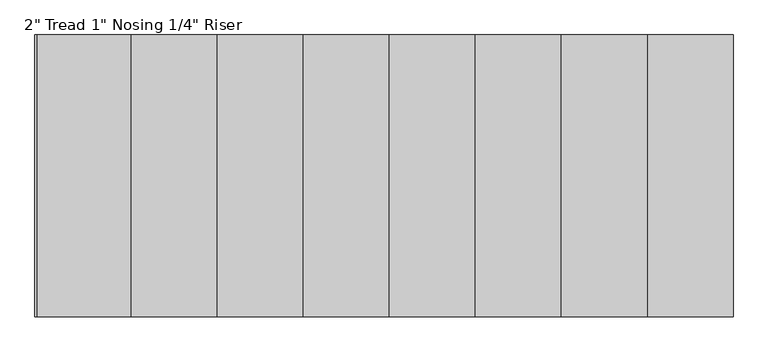
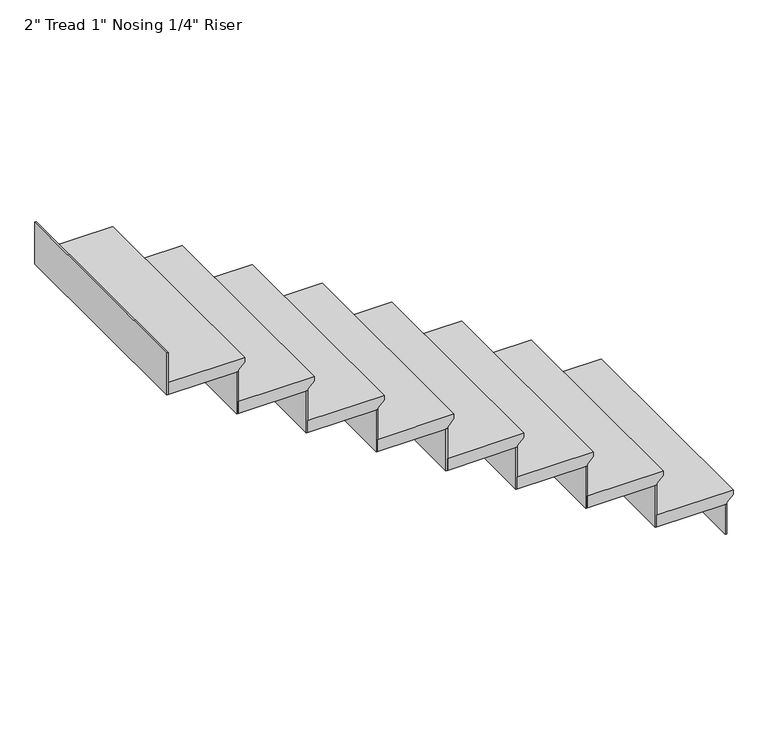
"""IFC4 building model written with IfcOpenShell, lengths in millimetres: stair flight geometry."""

from ifc_helpers import new_model, si_unit, origin, place, context, project, spatial, faceted_brep, source, transform, mapped, element, save


def stair_flight_c7deb699(model_context):
    return source(origin(), model_context, "Body", "Brep", [
        faceted_brep([(-3242.7473712, -4870.057676, 3359.15), (-3242.7473712, -4870.057676, 3378.2), (-3242.7473712, -5784.457676, 3378.2), (-3242.7473712, -5784.457676, 3359.15), (-3268.1473712, -4870.057676, 3333.75), (-3268.1473712, -5784.457676, 3333.75), (-3547.5473712, -4870.057676, 3378.2), (-3547.5473712, -5784.457676, 3378.2), (-3268.1473712, -5784.457676, 3327.4), (-3547.5473712, -5784.457676, 3327.4), (-3547.5473712, -4870.057676, 3327.4), (-3268.1473712, -4870.057676, 3327.4)], [[[0, 1, 2, 3]], [[4, 0, 3, 5]], [[2, 1, 6, 7]], [[8, 9, 10, 11]], [[2, 7, 9, 8, 5, 3]], [[8, 11, 4, 5]], [[6, 1, 0, 4, 11, 10]], [[7, 6, 10, 9]]]),
        faceted_brep([(-3268.1473712, -4870.057676, 3327.4), (-3268.1473712, -4870.057676, 3200.4), (-3274.4973712, -4870.057676, 3200.4), (-3274.4973712, -4870.057676, 3327.4), (-3268.1473712, -5784.457676, 3327.4), (-3274.4973712, -5784.457676, 3327.4), (-3274.4973712, -5784.457676, 3200.4), (-3268.1473712, -5784.457676, 3200.4)], [[[0, 1, 2, 3]], [[4, 5, 6, 7]], [[1, 0, 4, 7]], [[2, 1, 7, 6]], [[3, 2, 6, 5]], [[0, 3, 5, 4]]]),
        faceted_brep([(-5503.3473712, -4870.057676, 4749.8), (-5503.3473712, -4870.057676, 4572.0), (-5509.6973712, -4870.057676, 4572.0), (-5509.6973712, -4870.057676, 4749.8), (-5503.3473712, -5784.457676, 4749.8), (-5509.6973712, -5784.457676, 4749.8), (-5509.6973712, -5784.457676, 4572.0), (-5503.3473712, -5784.457676, 4572.0)], [[[0, 1, 2, 3]], [[4, 5, 6, 7]], [[1, 0, 4, 7]], [[2, 1, 7, 6]], [[3, 2, 6, 5]], [[0, 3, 5, 4]]]),
        faceted_brep([(-3547.5473712, -4870.057676, 3505.2), (-3547.5473712, -4870.057676, 3327.4), (-3553.8973712, -4870.057676, 3327.4), (-3553.8973712, -4870.057676, 3505.2), (-3547.5473712, -5784.457676, 3505.2), (-3553.8973712, -5784.457676, 3505.2), (-3553.8973712, -5784.457676, 3327.4), (-3547.5473712, -5784.457676, 3327.4)], [[[0, 1, 2, 3]], [[4, 5, 6, 7]], [[1, 0, 4, 7]], [[2, 1, 7, 6]], [[3, 2, 6, 5]], [[0, 3, 5, 4]]]),
        faceted_brep([(-3522.1473712, -5784.457676, 3556.0), (-3522.1473712, -4870.057676, 3556.0), (-3826.9473712, -4870.057676, 3556.0), (-3826.9473712, -5784.457676, 3556.0), (-3547.5473712, -5784.457676, 3505.2), (-3826.9473712, -5784.457676, 3505.2), (-3826.9473712, -4870.057676, 3505.2), (-3547.5473712, -4870.057676, 3505.2), (-3547.5473712, -5784.457676, 3511.55), (-3522.1473712, -5784.457676, 3536.95), (-3547.5473712, -4870.057676, 3511.55), (-3522.1473712, -4870.057676, 3536.95)], [[[0, 1, 2, 3]], [[4, 5, 6, 7]], [[0, 3, 5, 4, 8, 9]], [[4, 7, 10, 8]], [[2, 1, 11, 10, 7, 6]], [[3, 2, 6, 5]], [[11, 1, 0, 9]], [[10, 11, 9, 8]]]),
        faceted_brep([(-3826.9473712, -4870.057676, 3683.0), (-3826.9473712, -4870.057676, 3505.2), (-3833.2973712, -4870.057676, 3505.2), (-3833.2973712, -4870.057676, 3683.0), (-3826.9473712, -5784.457676, 3683.0), (-3833.2973712, -5784.457676, 3683.0), (-3833.2973712, -5784.457676, 3505.2), (-3826.9473712, -5784.457676, 3505.2)], [[[0, 1, 2, 3]], [[4, 5, 6, 7]], [[1, 0, 4, 7]], [[2, 1, 7, 6]], [[3, 2, 6, 5]], [[0, 3, 5, 4]]]),
        faceted_brep([(-3801.5473712, -5784.457676, 3733.8), (-3801.5473712, -4870.057676, 3733.8), (-4106.3473712, -4870.057676, 3733.8), (-4106.3473712, -5784.457676, 3733.8), (-3826.9473712, -5784.457676, 3683.0), (-4106.3473712, -5784.457676, 3683.0), (-4106.3473712, -4870.057676, 3683.0), (-3826.9473712, -4870.057676, 3683.0), (-3826.9473712, -5784.457676, 3689.35), (-3801.5473712, -5784.457676, 3714.75), (-3826.9473712, -4870.057676, 3689.35), (-3801.5473712, -4870.057676, 3714.75)], [[[0, 1, 2, 3]], [[4, 5, 6, 7]], [[0, 3, 5, 4, 8, 9]], [[4, 7, 10, 8]], [[2, 1, 11, 10, 7, 6]], [[3, 2, 6, 5]], [[11, 1, 0, 9]], [[10, 11, 9, 8]]]),
        faceted_brep([(-4106.3473712, -4870.057676, 3860.8), (-4106.3473712, -4870.057676, 3683.0), (-4112.6973712, -4870.057676, 3683.0), (-4112.6973712, -4870.057676, 3860.8), (-4106.3473712, -5784.457676, 3860.8), (-4112.6973712, -5784.457676, 3860.8), (-4112.6973712, -5784.457676, 3683.0), (-4106.3473712, -5784.457676, 3683.0)], [[[0, 1, 2, 3]], [[4, 5, 6, 7]], [[1, 0, 4, 7]], [[2, 1, 7, 6]], [[3, 2, 6, 5]], [[0, 3, 5, 4]]]),
        faceted_brep([(-4080.9473712, -5784.457676, 3911.6), (-4080.9473712, -4870.057676, 3911.6), (-4385.7473712, -4870.057676, 3911.6), (-4385.7473712, -5784.457676, 3911.6), (-4106.3473712, -5784.457676, 3860.8), (-4385.7473712, -5784.457676, 3860.8), (-4385.7473712, -4870.057676, 3860.8), (-4106.3473712, -4870.057676, 3860.8), (-4106.3473712, -5784.457676, 3867.15), (-4080.9473712, -5784.457676, 3892.55), (-4106.3473712, -4870.057676, 3867.15), (-4080.9473712, -4870.057676, 3892.55)], [[[0, 1, 2, 3]], [[4, 5, 6, 7]], [[0, 3, 5, 4, 8, 9]], [[4, 7, 10, 8]], [[2, 1, 11, 10, 7, 6]], [[3, 2, 6, 5]], [[11, 1, 0, 9]], [[10, 11, 9, 8]]]),
        faceted_brep([(-4385.7473712, -4870.057676, 4038.6), (-4385.7473712, -4870.057676, 3860.8), (-4392.0973712, -4870.057676, 3860.8), (-4392.0973712, -4870.057676, 4038.6), (-4385.7473712, -5784.457676, 4038.6), (-4392.0973712, -5784.457676, 4038.6), (-4392.0973712, -5784.457676, 3860.8), (-4385.7473712, -5784.457676, 3860.8)], [[[0, 1, 2, 3]], [[4, 5, 6, 7]], [[1, 0, 4, 7]], [[2, 1, 7, 6]], [[3, 2, 6, 5]], [[0, 3, 5, 4]]]),
        faceted_brep([(-4360.3473712, -5784.457676, 4089.4), (-4360.3473712, -4870.057676, 4089.4), (-4665.1473712, -4870.057676, 4089.4), (-4665.1473712, -5784.457676, 4089.4), (-4385.7473712, -5784.457676, 4038.6), (-4665.1473712, -5784.457676, 4038.6), (-4665.1473712, -4870.057676, 4038.6), (-4385.7473712, -4870.057676, 4038.6), (-4385.7473712, -5784.457676, 4044.95), (-4360.3473712, -5784.457676, 4070.35), (-4385.7473712, -4870.057676, 4044.95), (-4360.3473712, -4870.057676, 4070.35)], [[[0, 1, 2, 3]], [[4, 5, 6, 7]], [[0, 3, 5, 4, 8, 9]], [[4, 7, 10, 8]], [[2, 1, 11, 10, 7, 6]], [[3, 2, 6, 5]], [[11, 1, 0, 9]], [[10, 11, 9, 8]]]),
        faceted_brep([(-4665.1473712, -4870.057676, 4216.4), (-4665.1473712, -4870.057676, 4038.6), (-4671.4973712, -4870.057676, 4038.6), (-4671.4973712, -4870.057676, 4216.4), (-4665.1473712, -5784.457676, 4216.4), (-4671.4973712, -5784.457676, 4216.4), (-4671.4973712, -5784.457676, 4038.6), (-4665.1473712, -5784.457676, 4038.6)], [[[0, 1, 2, 3]], [[4, 5, 6, 7]], [[1, 0, 4, 7]], [[2, 1, 7, 6]], [[3, 2, 6, 5]], [[0, 3, 5, 4]]]),
        faceted_brep([(-4639.7473712, -5784.457676, 4267.2), (-4639.7473712, -4870.057676, 4267.2), (-4944.5473712, -4870.057676, 4267.2), (-4944.5473712, -5784.457676, 4267.2), (-4665.1473712, -5784.457676, 4216.4), (-4944.5473712, -5784.457676, 4216.4), (-4944.5473712, -4870.057676, 4216.4), (-4665.1473712, -4870.057676, 4216.4), (-4665.1473712, -5784.457676, 4222.75), (-4639.7473712, -5784.457676, 4248.15), (-4665.1473712, -4870.057676, 4222.75), (-4639.7473712, -4870.057676, 4248.15)], [[[0, 1, 2, 3]], [[4, 5, 6, 7]], [[0, 3, 5, 4, 8, 9]], [[4, 7, 10, 8]], [[2, 1, 11, 10, 7, 6]], [[3, 2, 6, 5]], [[11, 1, 0, 9]], [[10, 11, 9, 8]]]),
        faceted_brep([(-4944.5473712, -4870.057676, 4394.2), (-4944.5473712, -4870.057676, 4216.4), (-4950.8973712, -4870.057676, 4216.4), (-4950.8973712, -4870.057676, 4394.2), (-4944.5473712, -5784.457676, 4394.2), (-4950.8973712, -5784.457676, 4394.2), (-4950.8973712, -5784.457676, 4216.4), (-4944.5473712, -5784.457676, 4216.4)], [[[0, 1, 2, 3]], [[4, 5, 6, 7]], [[1, 0, 4, 7]], [[2, 1, 7, 6]], [[3, 2, 6, 5]], [[0, 3, 5, 4]]]),
        faceted_brep([(-4919.1473712, -5784.457676, 4445.0), (-4919.1473712, -4870.057676, 4445.0), (-5223.9473712, -4870.057676, 4445.0), (-5223.9473712, -5784.457676, 4445.0), (-4944.5473712, -5784.457676, 4394.2), (-5223.9473712, -5784.457676, 4394.2), (-5223.9473712, -4870.057676, 4394.2), (-4944.5473712, -4870.057676, 4394.2), (-4944.5473712, -5784.457676, 4400.55), (-4919.1473712, -5784.457676, 4425.95), (-4944.5473712, -4870.057676, 4400.55), (-4919.1473712, -4870.057676, 4425.95)], [[[0, 1, 2, 3]], [[4, 5, 6, 7]], [[0, 3, 5, 4, 8, 9]], [[4, 7, 10, 8]], [[2, 1, 11, 10, 7, 6]], [[3, 2, 6, 5]], [[11, 1, 0, 9]], [[10, 11, 9, 8]]]),
        faceted_brep([(-5223.9473712, -4870.057676, 4572.0), (-5223.9473712, -4870.057676, 4394.2), (-5230.2973712, -4870.057676, 4394.2), (-5230.2973712, -4870.057676, 4572.0), (-5223.9473712, -5784.457676, 4572.0), (-5230.2973712, -5784.457676, 4572.0), (-5230.2973712, -5784.457676, 4394.2), (-5223.9473712, -5784.457676, 4394.2)], [[[0, 1, 2, 3]], [[4, 5, 6, 7]], [[1, 0, 4, 7]], [[2, 1, 7, 6]], [[3, 2, 6, 5]], [[0, 3, 5, 4]]]),
        faceted_brep([(-5198.5473712, -5784.457676, 4622.8), (-5198.5473712, -4870.057676, 4622.8), (-5477.9473712, -4870.057676, 4622.8), (-5503.3473712, -4870.057676, 4622.8), (-5503.3473712, -5784.457676, 4622.8), (-5223.9473712, -5784.457676, 4572.0), (-5503.3473712, -5784.457676, 4572.0), (-5503.3473712, -4870.057676, 4572.0), (-5477.9473712, -4870.057676, 4572.0), (-5223.9473712, -4870.057676, 4572.0), (-5223.9473712, -5784.457676, 4578.35), (-5198.5473712, -5784.457676, 4603.75), (-5223.9473712, -4870.057676, 4578.35), (-5198.5473712, -4870.057676, 4603.75)], [[[0, 1, 2, 3, 4]], [[5, 6, 7, 8, 9]], [[0, 4, 6, 5, 10, 11]], [[5, 9, 12, 10]], [[2, 1, 13, 12, 9, 8]], [[3, 2, 8, 7]], [[4, 3, 7, 6]], [[13, 1, 0, 11]], [[12, 13, 11, 10]]]),
    ])


if __name__ == "__main__":
    model = new_model("IFC4")
    model_context = context("Model", 3, world=origin())
    ifc_project = project(units=[si_unit("LENGTHUNIT", "METRE", prefix="MILLI")], contexts=[model_context])
    site = spatial("IfcSite", under=ifc_project)
    building = spatial("IfcBuilding", under=site)
    placement = place(None, origin())
    stair_flight_shape = stair_flight_c7deb699(model_context)
    element("IfcStairFlight", 1, ObjectType="2\" Tread 1\" Nosing 1/4\" Riser", at=placement, inside=building, context=model_context, shape_type="MappedRepresentation", body=[
        mapped(stair_flight_shape, transform((0.0, 0.0, 0.0), x_axis=(1.0, 0.0, 0.0), y_axis=(0.0, 1.0, 0.0), z_axis=(0.0, 0.0, 1.0))),
    ])
    save(model, "model.ifc")
